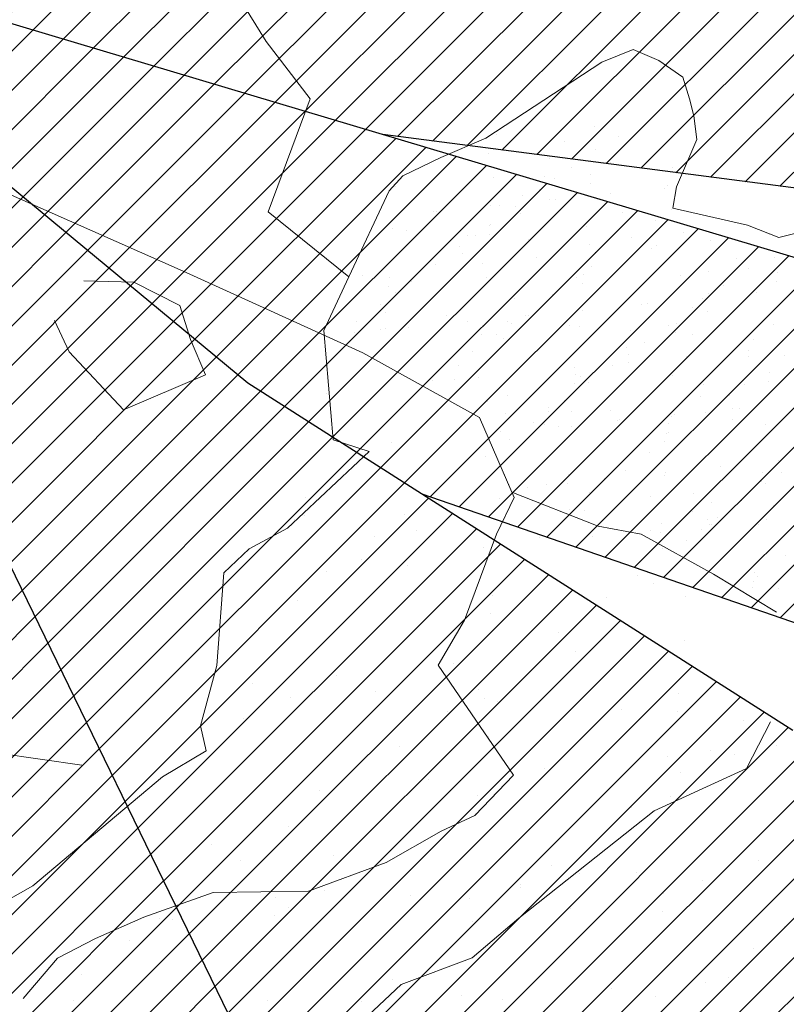
# Model space of a CAD drawing. Units: inches. Extents: x 1986 to 21484, y -1816 to 2016.
# Tile 68 of 85: x 3670.627 to 3674.872, y 1877.893 to 1883.347. Entities that reach past the tile are written whole.
import ezdxf

# ---------------------------------------------------------------- set-up
doc = ezdxf.new("R2010")
doc.units = ezdxf.units.IN
doc.layers.add('L-PLNT', color=84, linetype='Continuous', lineweight=13)
doc.layers.add('vfolhas', color=114, linetype='Continuous', lineweight=5)
for name, color, linetype in [('vfolha', 72, 'Continuous'), ('vfolha2', 110, 'Continuous'), ('vfolhas2', 102, 'Continuous')]:
    doc.layers.add(name, color=color, linetype=linetype)
pattern_1 = [(45, (-2446.5133113, 50.986076), (-0.004419417382, 0.004419417382), [])]

# ---------------------------------------------------------------- blocks, each defined once
blk = doc.blocks.new('arbusto_PB_verde_grande')
at = {"layer": 'vfolha2'}
h = blk.add_hatch(dxfattribs=at)
h.set_pattern_fill('ANSI31', color=256, scale=0.05, style=0)
h.set_pattern_definition(pattern_1)
h.paths.add_polyline_path([(0.02944, 0.35651), (0.00028, 0.09048), (0.02625, -0.03934), (0.047, 0.06233), (0.06189, 0.09731), (0.09372, 0.26573), (0.09955, 0.43473), (0.08789, 0.61313), (0.0645, 0.72266), (0.04988, 0.6851), (0.0236, 0.51294)])
h.paths.add_polyline_path([(0.30106, 0.43789), (0.14225, 0.24871), (0.26685, 0.30022)])
h.paths.add_polyline_path([(0.37995, 0.22817), (0.23697, 0.15193), (0.18428, 0.09364), (0.11122, 0.04358), (0.02625, -0.03934), (0.28061, 0.04667), (0.36829, 0.07798), (0.46756, 0.11239), (0.61068, 0.19376), (0.71585, 0.27823), (0.55813, 0.25948)])
h.paths.add_polyline_path([(0.56101, -0.29441), (0.72752, -0.32573), (0.59024, -0.2412), (0.42962, -0.15982), (0.02625, -0.03934), (0.14922, -0.14107), (0.18838, -0.16604), (0.41501, -0.24435)])
h.paths.add_polyline_path([(-0.27429, -0.44776), (-0.30352, -0.72628), (-0.23923, -0.64175), (-0.15457, -0.45716), (0.02625, -0.03934), (-0.16328, -0.25376)])
h.paths.add_polyline_path([(-0.51963, -0.24744), (-0.67736, -0.32573), (-0.59558, -0.35072), (-0.40574, -0.32882), (-0.21007, -0.20995), (0.02625, -0.03934), (-0.14874, -0.06595), (-0.31518, -0.09101), (-0.41452, -0.15048)])
h.paths.add_polyline_path([(-0.52546, 0.25007), (-0.70947, 0.24698), (-0.51963, 0.1093), (-0.32979, 0.02167), (-0.07567, -0.0128), (-0.04234, -0.02148), (-0.35024, 0.1312)])
h = blk.add_hatch(dxfattribs=at)
h.set_pattern_fill('ANSI31', color=256, scale=0.05, style=0)
h.set_pattern_definition(pattern_1)
h.paths.add_polyline_path([(-0.18963, 0.29704), (-0.08553, 0.20192), (-0.10785, 0.25007), (-0.13202, 0.31865), (-0.25096, 0.48479), (-0.44952, 0.5505), (-0.37946, 0.43789)])
h.paths.add_polyline_path([(0.07911, -0.4071), (0.08214, -0.50631), (0.17255, -0.6355), (0.18428, -0.44151), (0.14904, -0.29177), (0.02625, -0.03934), (0.03527, -0.25376)])
at = {"layer": 'vfolhas'}
h = blk.add_hatch(dxfattribs=at)
h.set_pattern_fill('ANSI31', color=256, scale=0.05, style=0)
h.set_pattern_definition(pattern_1)
h.paths.add_polyline_path([(-0.07279, 0.50669), (-0.18085, 0.65063), (-0.2334, 0.67253), (-0.20712, 0.53176), (-0.10785, 0.25007), (0.02625, -0.03934), (0.00028, 0.09048), (0.00816, 0.16241), (-0.04939, 0.29079)])
h.paths.add_polyline_path([(0.09902, 0.41929), (0.09372, 0.26573), (0.07906, 0.18814), (0.15506, 0.36901), (0.26606, 0.5505), (0.28356, 0.63504), (0.2485, 0.68819), (0.25145, 0.63504), (0.20178, 0.54426)])
h.paths.add_polyline_path([(0.12295, 0.24073), (0.047, 0.06233), (0.02625, -0.03934), (0.11122, 0.04358), (0.18428, 0.09364), (0.27478, 0.19376), (0.3215, 0.25323), (0.44129, 0.38467), (0.47634, 0.57866), (0.41789, 0.45347), (0.28939, 0.30954)])
h.paths.add_polyline_path([(0.58145, -0.03779), (0.70707, 0.01536), (0.78591, 0.04667), (0.74796, 0.06549), (0.62818, 0.08423), (0.52595, 0.09048), (0.39745, 0.04358), (0.02625, -0.03934), (0.25728, -0.03154), (0.43834, -0.0347)])
h.paths.add_polyline_path([(0.52022, -0.03647), (0.43834, -0.0347), (0.25728, -0.03154), (0.02625, -0.03934), (0.17964, -0.08515), (0.53768, -0.13167), (0.69541, -0.15357), (0.78591, -0.07852), (0.70413, -0.10042)])
h.paths.add_polyline_path([(0.27189, -0.21929), (0.14922, -0.14107), (0.02625, -0.03934), (0.15794, -0.31007), (0.29522, -0.42585), (0.41789, -0.49157), (0.56396, -0.56669), (0.5114, -0.48532), (0.39456, -0.34139)])
h.paths.add_polyline_path([(-0.05818, -0.47591), (-0.02312, -0.61984), (0.047, -0.80134), (0.08494, -0.59794), (0.07911, -0.4071), (0.03527, -0.25376), (0.02625, -0.03934), (-0.03773, -0.26001)])
h.paths.add_polyline_path([(-0.24218, 0.14054), (-0.11073, 0.06858), (0.02625, -0.03934), (-0.04235, 0.10871), (-0.21007, 0.23757), (-0.36485, 0.33145), (-0.47874, 0.40341), (-0.54303, 0.46288), (-0.49041, 0.33145), (-0.39408, 0.22192)])
at = {"layer": 'vfolha'}
blk.add_line((0.53768, -0.13167), (0.17964, -0.08515), dxfattribs=at)
at = {"layer": 'vfolha2'}
for p, q in [((0.42962, -0.15982), (0.02625, -0.03934)), ((0.02625, -0.03934), (0.15794, -0.31007)), ((0.18838, -0.16604), (0.41501, -0.24435))]:
    blk.add_line(p, q, dxfattribs=at)
at = {"layer": 'vfolhas2'}
for p, q in [((0.14922, -0.14107), (0.02625, -0.03934)), ((0.27189, -0.21929), (0.14922, -0.14107))]:
    blk.add_line(p, q, dxfattribs=at)
blk = doc.blocks.new('PLANT-SHRUB')
for p, q in [((2163.5458, 1898.0881), (2163.5458, 1898.0881)), ((2163.9638, 1898.0837), (2163.9638, 1898.0837)), ((2163.7538, 1898.0607), (2163.7538, 1898.0607)), ((2164.0787, 1898.0179), (2164.0787, 1898.0179)), ((2164.3302, 1897.8842), (2164.3302, 1897.8842)), ((2163.3996, 1897.7273), (2163.3996, 1897.7273)), ((2164.4791, 1897.6884), (2164.4791, 1897.6884)), ((2163.705, 1897.594), (2163.705, 1897.594)), ((2163.9825, 1897.5656), (2163.9825, 1897.5656)), ((2163.9088, 1897.4981), (2163.9088, 1897.4981)), ((2163.1007, 1897.3074), (2162.8262, 1897.2106)), ((2162.8925, 1897.327), (2162.8925, 1897.327)), ((2163.6336, 1897.1299), (2163.1007, 1897.3074)), ((2163.9387, 1897.3136), (2163.9387, 1897.3136)), ((2164.9611, 1897.3185), (2164.9611, 1897.3185)), ((2163.0982, 1897.2075), (2163.0982, 1897.2075)), ((2164.3428, 1897.2052), (2164.3428, 1897.2052)), ((2165.1103, 1897.1473), (2165.1103, 1897.1473)), ((2162.9297, 1897.1001), (2162.9297, 1897.1001)), ((2163.1773, 1897.1018), (2163.1773, 1897.1018)), ((2163.511, 1897.1336), (2163.511, 1897.1336)), ((2164.5862, 1897.0492), (2163.6336, 1897.1299)), ((2164.1743, 1897.0979), (2164.1743, 1897.0979)), ((2163.3853, 1897.0744), (2163.3853, 1897.0744)), ((2163.7102, 1897.0316), (2163.7102, 1897.0316)), ((2164.9253, 1897.0331), (2164.5862, 1897.0492)), ((2165.3128, 1896.8718), (2164.9253, 1897.0331)), ((2163.3745, 1896.9572), (2163.3745, 1896.9572)), ((2164.2531, 1896.9602), (2164.2531, 1896.9602)), ((2164.4611, 1896.9328), (2164.4611, 1896.9328)), ((2164.4539, 1896.9183), (2164.4539, 1896.9183)), ((2164.7861, 1896.89), (2164.7861, 1896.89)), ((2165.3128, 1896.8718), (2165.3128, 1896.8718)), ((2165.8457, 1896.8718), (2165.3128, 1896.8718)), ((2163.1633, 1896.815), (2163.1633, 1896.815)), ((2165.3289, 1896.8185), (2165.3289, 1896.8185)), ((2162.4964, 1896.3984), (2162.3874, 1896.7903)), ((2164.7125, 1896.7828), (2164.7125, 1896.7828)), ((2165.537, 1896.7911), (2165.537, 1896.7911)), ((2162.2877, 1896.7015), (2162.2877, 1896.7015)), ((2163.0897, 1896.7475), (2163.0897, 1896.7475)), ((2162.1375, 1896.5955), (2162.1375, 1896.5955)), ((2162.1375, 1896.5955), (2162.1375, 1896.5955)), ((2162.3918, 1896.6008), (2162.3918, 1896.6008)), ((2163.3822, 1896.5932), (2163.3822, 1896.5932)), ((2162.3251, 1896.5476), (2162.3251, 1896.5476)), ((2162.3276, 1896.5763), (2162.3276, 1896.5763)), ((2162.362, 1896.5813), (2162.362, 1896.5813)), ((2162.8673, 1896.5569), (2162.8673, 1896.5569)), ((2163.9135, 1896.5435), (2163.9135, 1896.5435)), ((2164.6268, 1896.5909), (2164.6268, 1896.5909)), ((2164.9359, 1896.5484), (2164.9359, 1896.5484)), ((2163.9528, 1895.7227), (2164.0665, 1896.4531)), ((2164.0665, 1896.4531), (2164.3751, 1896.4694)), ((2164.0665, 1896.4531), (2164.0665, 1896.4531)), ((2164.3648, 1896.4642), (2164.3648, 1896.4642)), ((2164.3751, 1896.4694), (2164.5701, 1896.4044)), ((2164.3751, 1896.4694), (2164.3751, 1896.4694)), ((2165.914, 1896.432), (2165.914, 1896.432)), ((2162.074, 1896.3762), (2162.074, 1896.3762)), ((2162.638, 1895.9629), (2162.4964, 1896.3984)), ((2162.6919, 1896.383), (2162.6919, 1896.383)), ((2164.2911, 1896.3967), (2164.2911, 1896.3967)), ((2164.5701, 1896.4044), (2164.9112, 1896.3233)), ((2161.9957, 1896.3485), (2161.9957, 1896.3485)), ((2162.1262, 1896.3653), (2162.1262, 1896.3653)), ((2164.9112, 1896.3233), (2165.3335, 1896.1447)), ((2161.837, 1896.2434), (2161.837, 1896.2434)), ((2161.941, 1896.2297), (2161.941, 1896.2297)), ((2161.941, 1896.2297), (2161.941, 1896.2297)), ((2161.941, 1896.2297), (2161.941, 1896.2297)), ((2161.8038, 1896.1888), (2161.8038, 1896.1888)), ((2161.9155, 1896.1722), (2161.9155, 1896.1722)), ((2161.9524, 1896.206), (2161.9524, 1896.206)), ((2162.1035, 1896.2083), (2162.1035, 1896.2083)), ((2162.2659, 1896.187), (2162.2659, 1896.187)), ((2162.2659, 1896.187), (2162.2659, 1896.187)), ((2162.315, 1896.1913), (2162.315, 1896.1913)), ((2162.3269, 1896.1822), (2162.3269, 1896.1822)), ((2162.3269, 1896.1822), (2162.3269, 1896.1822)), ((2162.3749, 1896.1726), (2162.3749, 1896.1726)), ((2162.4789, 1896.1589), (2162.4789, 1896.1589)), ((2162.7754, 1896.2067), (2162.7754, 1896.2067)), ((2163.3493, 1896.1871), (2163.3493, 1896.1871)), ((2164.0201, 1896.2044), (2164.0201, 1896.2044)), ((2165.2647, 1896.2022), (2165.2647, 1896.2022)), ((2162.2304, 1896.1004), (2162.2304, 1896.1004)), ((2162.3146, 1896.1541), (2162.3146, 1896.1541)), ((2162.8088, 1896.1155), (2162.8088, 1896.1155)), ((2164.4287, 1896.1482), (2164.4287, 1896.1482)), ((2165.3335, 1896.1447), (2165.7234, 1895.7876)), ((2165.3335, 1896.1447), (2165.3335, 1896.1447)), ((2165.4749, 1896.1348), (2165.4749, 1896.1348)), ((2165.5662, 1896.1134), (2165.5662, 1896.1134)), ((2162.3441, 1896.0644), (2162.3441, 1896.0644)), ((2162.3441, 1896.0644), (2162.3441, 1896.0644)), ((2162.6069, 1896.0993), (2162.6069, 1896.0993)), ((2163.0168, 1896.0881), (2163.0168, 1896.0881)), ((2163.8515, 1896.097), (2163.8515, 1896.097)), ((2165.0962, 1896.0948), (2165.0962, 1896.0948)), ((2165.4926, 1896.0459), (2165.4926, 1896.0459)), ((2162.0614, 1895.9911), (2162.0614, 1895.9911)), ((2162.2705, 1895.9968), (2162.2705, 1895.9968)), ((2162.2705, 1895.9968), (2162.2705, 1895.9968)), ((2162.5163, 1895.9968), (2162.5163, 1895.9968)), ((2162.5531, 1896.0306), (2162.5531, 1896.0306)), ((2163.3417, 1896.0453), (2163.3417, 1896.0453)), ((2163.8933, 1896.0322), (2163.8933, 1896.0322)), ((2161.7166, 1895.99), (2161.7166, 1895.99)), ((2162.5845, 1895.9845), (2162.5845, 1895.9845)), ((2162.7797, 1895.7669), (2162.638, 1895.9629)), ((2163.8846, 1895.9739), (2163.8846, 1895.9739)), ((2164.0926, 1895.9465), (2164.0926, 1895.9465)), ((2164.4176, 1895.9037), (2164.4176, 1895.9037)), ((2161.5428, 1895.8307), (2161.5428, 1895.8307)), ((2161.8343, 1895.8481), (2161.8343, 1895.8481)), ((2162.4566, 1895.847), (2162.4566, 1895.847)), ((2164.9604, 1895.8322), (2164.9604, 1895.8322)), ((2161.3813, 1895.786), (2161.3813, 1895.786)), ((2161.506, 1895.7969), (2161.506, 1895.7969)), ((2161.7627, 1895.8257), (2161.7627, 1895.8257)), ((2161.7627, 1895.8257), (2161.7627, 1895.8257)), ((2161.7912, 1895.8038), (2161.7912, 1895.8038)), ((2162.3024, 1895.8062), (2162.3024, 1895.8062)), ((2162.3174, 1895.8146), (2162.3174, 1895.8146)), ((2162.8421, 1895.7868), (2162.8421, 1895.7868)), ((2163.8883, 1895.7734), (2163.8883, 1895.7734)), ((2164.9107, 1895.7783), (2164.9107, 1895.7783)), ((2165.1685, 1895.8048), (2165.1685, 1895.8048)), ((2165.7234, 1895.7876), (2166.097, 1895.6253)), ((2165.7234, 1895.7876), (2165.7234, 1895.7876)), ((2161.6527, 1895.7503), (2161.6527, 1895.7503)), ((2161.7568, 1895.7366), (2161.7568, 1895.7366)), ((2162.9997, 1895.3027), (2162.7797, 1895.7669)), ((2163.6766, 1895.6415), (2163.9528, 1895.7227)), ((2165.4934, 1895.7621), (2165.4934, 1895.7621)), ((2165.9902, 1895.7395), (2165.9902, 1895.7395)), ((2161.9192, 1895.7152), (2161.9192, 1895.7152)), ((2162.1906, 1895.6795), (2162.1906, 1895.6795)), ((2162.2947, 1895.6658), (2162.2947, 1895.6658)), ((2163.5456, 1895.7136), (2163.5456, 1895.7136)), ((2165.0948, 1895.6814), (2165.0948, 1895.6814)), ((2166.0363, 1895.6906), (2166.0363, 1895.6906)), ((2166.694, 1895.6951), (2166.694, 1895.6951)), ((2161.3071, 1895.6147), (2161.3071, 1895.6147)), ((2161.5091, 1895.6255), (2161.5091, 1895.6255)), ((2161.5309, 1895.6548), (2161.5309, 1895.6548)), ((2161.8727, 1895.6323), (2161.8727, 1895.6323)), ((2161.8727, 1895.6323), (2161.8727, 1895.6323)), ((2162.1067, 1895.6215), (2162.1067, 1895.6215)), ((2162.1435, 1895.6553), (2162.1435, 1895.6553)), ((2162.1532, 1895.6537), (2162.1532, 1895.6537)), ((2162.4571, 1895.6444), (2162.4571, 1895.6444)), ((2162.7756, 1895.6526), (2162.7756, 1895.6526)), ((2163.2218, 1895.4143), (2163.6766, 1895.6415)), ((2163.4719, 1895.6461), (2163.4719, 1895.6461)), ((2166.097, 1895.6253), (2166.3732, 1895.5279)), ((2166.2443, 1895.6632), (2166.2443, 1895.6632)), ((2166.5692, 1895.6204), (2166.5692, 1895.6204)), ((2161.4467, 1895.6012), (2161.4467, 1895.6012)), ((2161.8148, 1895.5947), (2161.8148, 1895.5947)), ((2161.8148, 1895.5947), (2161.8148, 1895.5947)), ((2162.0488, 1895.6061), (2162.0488, 1895.6061)), ((2162.069, 1895.6), (2162.069, 1895.6)), ((2162.5719, 1895.5994), (2162.5719, 1895.5994)), ((2162.6913, 1895.5989), (2162.6913, 1895.5989)), ((2162.7286, 1895.6086), (2162.7286, 1895.6086)), ((2162.8326, 1895.595), (2162.8326, 1895.595)), ((2163.0594, 1895.5924), (2163.0594, 1895.5924)), ((2164.304, 1895.5901), (2164.304, 1895.5901)), ((2165.5486, 1895.5879), (2165.5486, 1895.5879)), ((2166.7933, 1895.5856), (2166.7933, 1895.5856)), ((2166.3732, 1895.5279), (2166.6006, 1895.463)), ((2160.5943, 1895.4848), (2160.9564, 1895.2869)), ((2161.1332, 1895.4554), (2161.1332, 1895.4554)), ((2162.7074, 1895.4461), (2162.7074, 1895.4461)), ((2162.7443, 1895.4799), (2162.7443, 1895.4799)), ((2166.6006, 1895.463), (2166.893, 1895.4955)), ((2166.893, 1895.4955), (2166.893, 1895.4955)), ((2161.0964, 1895.4216), (2161.0964, 1895.4216)), ((2161.2555, 1895.4254), (2161.2555, 1895.4254)), ((2161.2555, 1895.4254), (2161.2555, 1895.4254)), ((2161.2555, 1895.4254), (2161.2555, 1895.4254)), ((2161.7786, 1895.4187), (2161.7786, 1895.4187)), ((2161.9078, 1895.4393), (2161.9078, 1895.4393)), ((2162.2898, 1895.4212), (2162.2898, 1895.4212)), ((2162.3017, 1895.4121), (2162.3017, 1895.4121)), ((2162.3017, 1895.4121), (2162.3017, 1895.4121)), ((2162.8295, 1895.4017), (2162.8295, 1895.4017)), ((2163.0106, 1895.3331), (2163.2218, 1895.4143)), ((2163.3241, 1895.417), (2163.3241, 1895.417)), ((2161.0506, 1895.3488), (2161.0506, 1895.3488)), ((2161.6729, 1895.3477), (2161.6729, 1895.3477)), ((2162.2952, 1895.3466), (2162.2952, 1895.3466)), ((2162.9175, 1895.3454), (2162.9175, 1895.3454)), ((2164.4036, 1895.3781), (2164.4036, 1895.3781)), ((2164.7471, 1895.3628), (2164.7471, 1895.3628)), ((2160.9564, 1895.2869), (2161.0356, 1895.1173)), ((2161.0346, 1895.3143), (2161.0346, 1895.3143)), ((2161.1971, 1895.2929), (2161.1971, 1895.2929)), ((2161.525, 1895.3137), (2161.525, 1895.3137)), ((2161.525, 1895.3137), (2161.525, 1895.3137)), ((2162.8481, 1894.8786), (2163.0106, 1895.3331)), ((2162.8481, 1894.8786), (2162.9997, 1895.3027)), ((2164.6734, 1895.2953), (2164.6734, 1895.2953)), ((2160.9853, 1895.238), (2160.9853, 1895.238)), ((2161.3645, 1895.2708), (2161.3645, 1895.2708)), ((2161.3645, 1895.2708), (2161.3645, 1895.2708)), ((2161.4513, 1895.2462), (2161.4513, 1895.2462)), ((2161.4513, 1895.2462), (2161.4513, 1895.2462)), ((2161.4685, 1895.2571), (2161.4685, 1895.2571)), ((2161.4965, 1895.2405), (2161.4965, 1895.2405)), ((2161.5725, 1895.2434), (2161.5725, 1895.2434)), ((2161.5725, 1895.2434), (2161.5725, 1895.2434)), ((2161.5725, 1895.2434), (2161.5725, 1895.2434)), ((2161.6971, 1895.2462), (2161.6971, 1895.2462)), ((2161.7339, 1895.28), (2161.7339, 1895.28)), ((2162.5085, 1895.2639), (2162.5085, 1895.2639)), ((2163.0741, 1895.2815), (2163.0741, 1895.2815)), ((2161.208, 1895.2081), (2161.208, 1895.2081)), ((2161.208, 1895.2081), (2161.208, 1895.2081)), ((2161.735, 1895.2221), (2161.735, 1895.2221)), ((2161.8974, 1895.2007), (2161.8974, 1895.2007)), ((2161.8974, 1895.2007), (2161.8974, 1895.2007)), ((2162.0064, 1895.1863), (2162.0064, 1895.1863)), ((2162.0362, 1895.221), (2162.0362, 1895.221)), ((2162.4526, 1895.2059), (2162.4526, 1895.2059)), ((2162.4526, 1895.2059), (2162.4526, 1895.2059)), ((2162.5593, 1895.2144), (2162.5593, 1895.2144)), ((2163.6973, 1895.2036), (2163.6973, 1895.2036)), ((2164.9419, 1895.2013), (2164.9419, 1895.2013)), ((2165.1435, 1895.0672), (2165.2147, 1895.1892)), ((2165.2147, 1895.1892), (2165.4893, 1895.1282)), ((2161.3695, 1895.1544), (2161.3695, 1895.1544)), ((2161.9919, 1895.1533), (2161.9919, 1895.1533)), ((2162.1104, 1895.1726), (2162.1104, 1895.1726)), ((2162.2729, 1895.1512), (2162.2729, 1895.1512)), ((2162.4403, 1895.1292), (2162.4403, 1895.1292)), ((2162.4403, 1895.1292), (2162.4403, 1895.1292)), ((2162.6142, 1895.1522), (2162.6142, 1895.1522)), ((2165.4893, 1895.1282), (2166.4251, 1895.0774)), ((2161.0356, 1895.1173), (2161.2731, 1894.7669)), ((2161.2853, 1895.1007), (2161.2853, 1895.1007)), ((2161.9076, 1895.0996), (2161.9076, 1895.0996)), ((2162.2841, 1895.0985), (2162.2841, 1895.0985)), ((2162.2841, 1895.0985), (2162.2841, 1895.0985)), ((2162.2978, 1895.0708), (2162.2978, 1895.0708)), ((2162.3347, 1895.1046), (2162.3347, 1895.1046)), ((2162.5299, 1895.0985), (2162.5299, 1895.0985)), ((2162.5443, 1895.1155), (2162.5443, 1895.1155)), ((2162.6483, 1895.1018), (2162.6483, 1895.1018)), ((2162.6483, 1895.1018), (2162.6483, 1895.1018)), ((2162.6483, 1895.1018), (2162.6483, 1895.1018)), ((2162.8108, 1895.0804), (2162.8108, 1895.0804)), ((2163.5287, 1895.0962), (2163.5287, 1895.0962)), ((2164.7734, 1895.094), (2164.7734, 1895.094)), ((2164.8485, 1894.8843), (2165.1435, 1895.0672)), ((2166.4251, 1895.0774), (2167.1371, 1894.9046)), ((2161.2429, 1895.0404), (2161.2429, 1895.0404)), ((2161.4982, 1895.064), (2161.4982, 1895.064)), ((2161.7375, 1895.0556), (2161.7375, 1895.0556)), ((2161.7375, 1895.0556), (2161.7375, 1895.0556)), ((2161.766, 1895.0337), (2161.766, 1895.0337)), ((2162.2772, 1895.0361), (2162.2772, 1895.0361)), ((2162.817, 1895.0167), (2162.817, 1895.0167)), ((2162.817, 1895.0167), (2162.817, 1895.0167)), ((2162.817, 1895.0167), (2162.817, 1895.0167)), ((2162.9733, 1895.059), (2162.9733, 1895.059)), ((2162.7264, 1894.9629), (2162.7264, 1894.9629)), ((2162.7264, 1894.9629), (2162.7264, 1894.9629)), ((2163.5161, 1894.9876), (2163.5161, 1894.9876)), ((2163.7242, 1894.9602), (2163.7242, 1894.9602)), ((2163.8631, 1895.0033), (2163.8631, 1895.0033)), ((2161.3243, 1894.9046), (2161.3243, 1894.9046)), ((2164.0491, 1894.9174), (2164.0491, 1894.9174)), ((2164.2756, 1894.9308), (2164.2756, 1894.9308)), ((2161.2875, 1894.8709), (2161.2875, 1894.8709)), ((2161.4839, 1894.8554), (2161.4839, 1894.8554)), ((2161.5115, 1894.8473), (2161.5115, 1894.8473)), ((2162.0989, 1894.8886), (2162.0989, 1894.8886)), ((2162.1338, 1894.8462), (2162.1338, 1894.8462)), ((2162.6528, 1894.8954), (2162.6528, 1894.8954)), ((2162.6528, 1894.8954), (2162.6528, 1894.8954)), ((2163.0739, 1894.1758), (2162.8481, 1894.8786)), ((2164.4688, 1894.5366), (2164.8485, 1894.8843)), ((2164.8485, 1894.8843), (2164.8485, 1894.8843)), ((2162.0237, 1894.836), (2162.0237, 1894.836)), ((2162.5467, 1894.8293), (2162.5467, 1894.8293)), ((2162.7561, 1894.845), (2162.7561, 1894.845)), ((2161.2731, 1894.7669), (2161.177, 1894.6934)), ((2161.2842, 1894.764), (2161.2842, 1894.764)), ((2161.3883, 1894.7503), (2161.3883, 1894.7503)), ((2166.4276, 1893.9579), (2165.771, 1894.7754)), ((2161.177, 1894.6934), (2160.9168, 1894.5803)), ((2161.5507, 1894.7289), (2161.5507, 1894.7289)), ((2161.8222, 1894.6932), (2161.8222, 1894.6932)), ((2161.8882, 1894.6955), (2161.8882, 1894.6955)), ((2161.9251, 1894.7293), (2161.9251, 1894.7293)), ((2162.6997, 1894.7132), (2162.6997, 1894.7132)), ((2161.2081, 1894.654), (2161.2081, 1894.654)), ((2161.2304, 1894.6553), (2161.2304, 1894.6553)), ((2161.2304, 1894.6553), (2161.2304, 1894.6553)), ((2161.2304, 1894.6553), (2161.2304, 1894.6553)), ((2161.7534, 1894.6486), (2161.7534, 1894.6486)), ((2161.8305, 1894.6529), (2161.8305, 1894.6529)), ((2161.9262, 1894.6795), (2161.9262, 1894.6795)), ((2162.0886, 1894.6581), (2162.0886, 1894.6581)), ((2162.2646, 1894.6511), (2162.2646, 1894.6511)), ((2162.2765, 1894.642), (2162.2765, 1894.642)), ((2162.2765, 1894.642), (2162.2765, 1894.642)), ((2162.4528, 1894.6518), (2162.4528, 1894.6518)), ((2162.8044, 1894.6316), (2162.8044, 1894.6316)), ((2163.2989, 1894.6469), (2163.2989, 1894.6469)), ((2160.9168, 1894.5803), (2160.8376, 1894.4729)), ((2161.1239, 1894.6003), (2161.1239, 1894.6003)), ((2161.492, 1894.5938), (2161.492, 1894.5938)), ((2161.492, 1894.5938), (2161.492, 1894.5938)), ((2161.7462, 1894.5992), (2161.7462, 1894.5992)), ((2162.3601, 1894.6224), (2162.3601, 1894.6224)), ((2162.3685, 1894.5981), (2162.3685, 1894.5981)), ((2162.4641, 1894.6087), (2162.4641, 1894.6087)), ((2162.6265, 1894.5873), (2162.6265, 1894.5873)), ((2162.7366, 1894.5916), (2162.7366, 1894.5916)), ((2162.7366, 1894.5916), (2162.7366, 1894.5916)), ((2163.4212, 1894.5976), (2164.0416, 1894.5976)), ((2163.4212, 1894.5976), (2163.4212, 1894.5976)), ((2163.5229, 1894.4146), (2163.4212, 1894.5976)), ((2163.9279, 1894.6122), (2163.9279, 1894.6122)), ((2163.9812, 1894.5893), (2163.9812, 1894.5893)), ((2164.0416, 1894.5976), (2164.2756, 1894.5366)), ((2162.255, 1894.5309), (2162.255, 1894.5309)), ((2162.255, 1894.5309), (2162.255, 1894.5309)), ((2162.489, 1894.5201), (2162.489, 1894.5201)), ((2162.5258, 1894.5539), (2162.5258, 1894.5539)), ((2162.898, 1894.5515), (2162.898, 1894.5515)), ((2163.8542, 1894.5446), (2163.8542, 1894.5446)), ((2164.2756, 1894.5366), (2164.4688, 1894.5366)), ((2160.8376, 1894.4729), (2160.7923, 1894.3882)), ((2161.4713, 1894.4704), (2161.4713, 1894.4704)), ((2161.6893, 1894.5132), (2161.6893, 1894.5132)), ((2162.0111, 1894.451), (2162.0111, 1894.451)), ((2162.5342, 1894.4443), (2162.5342, 1894.4443)), ((2163.1465, 1893.9369), (2163.5229, 1894.4146)), ((2160.7923, 1894.3882), (2160.7357, 1894.2751)), ((2161.3501, 1894.3469), (2161.3501, 1894.3469)), ((2161.4787, 1894.3202), (2161.4787, 1894.3202)), ((2161.5155, 1894.3539), (2161.5155, 1894.3539)), ((2161.9724, 1894.3458), (2161.9724, 1894.3458)), ((2162.2901, 1894.3379), (2162.2901, 1894.3379)), ((2162.5948, 1894.3446), (2162.5948, 1894.3446)), ((2160.7357, 1894.2751), (2160.7697, 1894.1168)), ((2160.7357, 1894.2751), (2160.7357, 1894.2751)), ((2161.2178, 1894.2703), (2161.2178, 1894.2703)), ((2161.7123, 1894.2855), (2161.7123, 1894.2855)), ((2161.7123, 1894.2855), (2161.7123, 1894.2855)), ((2161.7408, 1894.2636), (2161.7408, 1894.2636)), ((2162.252, 1894.266), (2162.252, 1894.266)), ((2162.7918, 1894.2466), (2162.7918, 1894.2466)), ((2162.7918, 1894.2466), (2162.7918, 1894.2466)), ((2162.7918, 1894.2466), (2162.7918, 1894.2466)), ((2161.3665, 1894.2358), (2161.3665, 1894.2358)), ((2161.5289, 1894.2144), (2161.5289, 1894.2144)), ((2161.5289, 1894.2144), (2161.5289, 1894.2144)), ((2161.6379, 1894.2), (2161.6379, 1894.2)), ((2161.9073, 1894.2123), (2161.9073, 1894.2123)), ((2161.9073, 1894.2123), (2161.9073, 1894.2123)), ((2162.1299, 1894.205), (2162.1299, 1894.205)), ((2162.1299, 1894.205), (2162.1299, 1894.205)), ((2163.3745, 1894.2028), (2163.3745, 1894.2028)), ((2161.2797, 1894.1379), (2161.2797, 1894.1379)), ((2161.6691, 1894.1525), (2161.6691, 1894.1525)), ((2161.7419, 1894.1863), (2161.7419, 1894.1863)), ((2161.8336, 1894.1448), (2161.8336, 1894.1448)), ((2161.8336, 1894.1448), (2161.8336, 1894.1448)), ((2161.9044, 1894.1649), (2161.9044, 1894.1649)), ((2162.0718, 1894.1429), (2162.0718, 1894.1429)), ((2162.0718, 1894.1429), (2162.0718, 1894.1429)), ((2162.0794, 1894.1448), (2162.0794, 1894.1448)), ((2162.1162, 1894.1785), (2162.1162, 1894.1785)), ((2162.2914, 1894.1514), (2162.2914, 1894.1514)), ((2162.8908, 1894.1625), (2162.8908, 1894.1625)), ((2162.9137, 1894.1502), (2162.9137, 1894.1502)), ((2163.4826, 1893.1809), (2163.0739, 1894.1758)), ((2160.7697, 1894.1168), (2160.8319, 1893.9755)), ((2161.4587, 1894.0854), (2161.4587, 1894.0854)), ((2161.5848, 1894.0988), (2161.5848, 1894.0988)), ((2161.9613, 1894.0977), (2161.9613, 1894.0977)), ((2161.9613, 1894.0977), (2161.9613, 1894.0977)), ((2162.1758, 1894.1292), (2162.1758, 1894.1292)), ((2162.2071, 1894.0977), (2162.2071, 1894.0977)), ((2162.2798, 1894.1155), (2162.2798, 1894.1155)), ((2162.2798, 1894.1155), (2162.2798, 1894.1155)), ((2162.2798, 1894.1155), (2162.2798, 1894.1155)), ((2162.4423, 1894.0941), (2162.4423, 1894.0941)), ((2162.8294, 1894.0965), (2162.8294, 1894.0965)), ((2161.9985, 1894.0659), (2161.9985, 1894.0659)), ((2162.5216, 1894.0592), (2162.5216, 1894.0592)), ((2162.6048, 1894.0727), (2162.6048, 1894.0727)), ((2162.6048, 1894.0727), (2162.6048, 1894.0727)), ((2162.7137, 1894.0584), (2162.7137, 1894.0584)), ((2162.8177, 1894.0447), (2162.8177, 1894.0447)), ((2163.0328, 1894.0617), (2163.0328, 1894.0617)), ((2160.8319, 1893.9755), (2161.0073, 1893.9077)), ((2162.7169, 1894.0032), (2162.7169, 1894.0032)), ((2162.9802, 1894.0233), (2162.9802, 1894.0233)), ((2161.8805, 1893.9625), (2161.8805, 1893.9625)), ((2162.6801, 1893.9694), (2162.6801, 1893.9694)), ((2162.8414, 1893.815), (2163.1465, 1893.9369)), ((2161.0073, 1893.9077), (2161.7632, 1893.7743)), ((2161.7283, 1893.8785), (2161.7283, 1893.8785)), ((2162.2395, 1893.881), (2162.2395, 1893.881)), ((2162.2513, 1893.8719), (2162.2513, 1893.8719)), ((2162.2513, 1893.8719), (2162.2513, 1893.8719)), ((2161.811, 1893.8453), (2161.811, 1893.8453)), ((2162.3532, 1893.6218), (2162.8414, 1893.815)), ((2162.4334, 1893.8442), (2162.4334, 1893.8442)), ((2162.7792, 1893.8615), (2162.7792, 1893.8615)), ((2162.8414, 1893.815), (2162.92, 1893.2475)), ((2162.8414, 1893.815), (2162.8414, 1893.815)), ((2161.7066, 1893.8032), (2161.7066, 1893.8032)), ((2161.7632, 1893.7743), (2162.0175, 1893.6828)), ((2162.4812, 1893.7871), (2162.4812, 1893.7871)), ((2162.0175, 1893.6828), (2162.2413, 1893.6117)), ((2163.7921, 1893.669), (2163.7182, 1893.4682)), ((2164.2561, 1893.4981), (2163.7921, 1893.669)), ((2162.2413, 1893.6117), (2162.3532, 1893.6218)), ((2162.3074, 1893.6278), (2162.3074, 1893.6278)), ((2164.2561, 1893.4981), (2164.2561, 1893.4981)), ((2164.2561, 1893.0589), (2164.2561, 1893.4981)), ((2163.7182, 1893.4682), (2163.6333, 1893.2907)), ((2163.6333, 1893.2907), (2163.731, 1893.0222)), ((2162.92, 1893.2475), (2162.3233, 1892.9494)), ((2163.9242, 1892.1391), (2163.4826, 1893.1809)), ((2164.1951, 1892.8758), (2164.2561, 1893.0589)), ((2163.731, 1893.0222), (2163.9264, 1892.827)), ((2162.3233, 1892.9494), (2162.2835, 1892.5519)), ((2162.2835, 1892.5519), (2162.1841, 1892.075)), ((2162.2835, 1892.5519), (2162.2835, 1892.5519))]:
    blk.add_line(p, q)

msp = doc.modelspace()

# ---------------------------------------------------------------- block references
at = {"layer": 'L-PLNT', "rotation": 223.1883365522388}
msp.add_blockref('PLANT-SHRUB', (3953.27, 4742.9646), dxfattribs=at)
at = {"layer": 'L-PLNT', "xscale": 24.60366729364114, "yscale": 24.60366729364114, "zscale": 24.60366729364114}
msp.add_blockref('arbusto_PB_verde_grande', (3668.2184, 1884.8051), dxfattribs=at)

doc.saveas('drawing.dxf')
